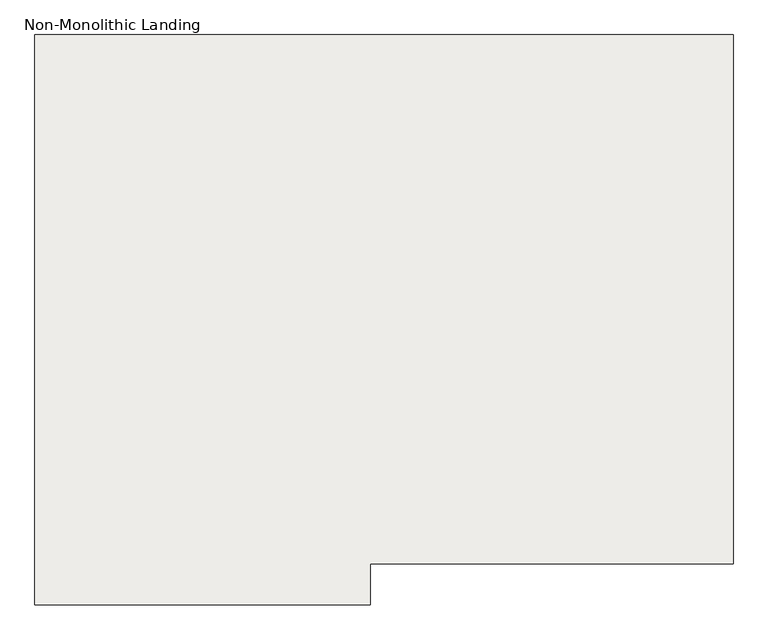
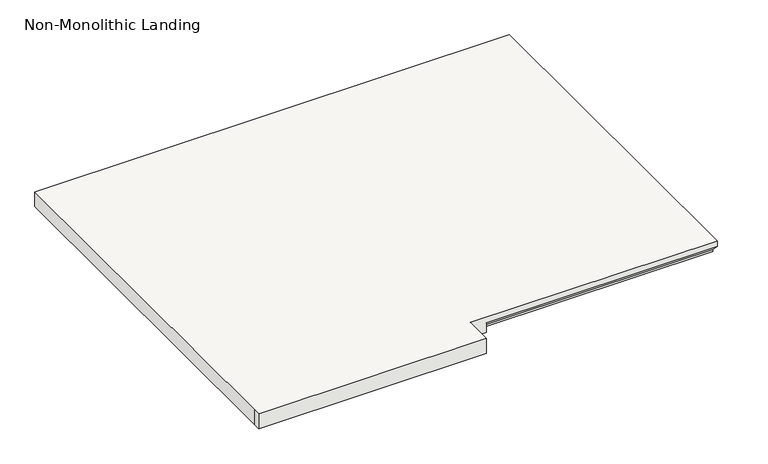
"""IFC4 building model written with IfcOpenShell, lengths in millimetres: slab geometry, Non-Monolithic Landing."""

from ifc_helpers import new_model, si_unit, origin, place, context, project, spatial, faceted_brep, source, transform, mapped, element, save


def non_monolithic_landing_83642a75(model_context):
    return source(origin(), model_context, "Body", "Brep", [
        faceted_brep([(-5330.5155596, 6109.0076853, 831.85), (-5330.5155596, 6083.6076853, 857.25), (-6072.1955596, 6083.6076853, 857.25), (-6072.1955596, 6109.0076853, 831.85), (-5330.5155596, 7239.3076853, 876.3), (-6854.5155596, 7239.3076853, 876.3), (-6854.5155596, 6020.1076853, 876.3), (-6854.5155596, 5994.7076853, 876.3), (-6122.9955596, 5994.7076853, 876.3), (-6122.9955596, 6020.1076853, 876.3), (-6122.9955596, 6083.6076853, 876.3), (-5330.5155596, 6083.6076853, 876.3), (-6072.1955596, 6109.0076853, 825.5), (-6072.1955596, 6083.6076853, 825.5), (-6122.9955596, 6083.6076853, 825.5), (-6122.9955596, 6020.1076853, 825.5), (-6122.9955596, 5994.7076853, 825.5), (-6854.5155596, 5994.7076853, 825.5), (-6854.5155596, 6020.1076853, 825.5), (-6854.5155596, 7239.3076853, 825.5), (-5330.5155596, 7239.3076853, 825.5), (-5330.5155596, 6109.0076853, 825.5)], [[[0, 1, 2, 3]], [[4, 5, 6, 7, 8, 9, 10, 11]], [[12, 13, 14, 15, 16, 17, 18, 19, 20, 21]], [[13, 12, 3, 2]], [[12, 21, 0, 3]], [[4, 11, 1, 0, 21, 20]], [[5, 4, 20, 19]], [[6, 5, 19, 18]], [[7, 6, 18, 17]], [[8, 7, 17, 16]], [[9, 8, 16, 15]], [[10, 9, 15, 14]], [[11, 10, 14, 13, 2, 1]]]),
    ])


if __name__ == "__main__":
    model = new_model("IFC4")
    model_context = context("Model", 3, world=origin())
    ifc_project = project(units=[si_unit("LENGTHUNIT", "METRE", prefix="MILLI")], contexts=[model_context])
    site = spatial("IfcSite", under=ifc_project)
    building = spatial("IfcBuilding", under=site)
    placement = place(None, origin())
    non_monolithic_landing_shape = non_monolithic_landing_83642a75(model_context)
    element("IfcSlab", 1, ObjectType="Non-Monolithic Landing", at=placement, inside=building, context=model_context, shape_type="MappedRepresentation", body=[
        mapped(non_monolithic_landing_shape, transform((0.0, 0.0, 0.0), x_axis=(1.0, 0.0, 0.0), y_axis=(0.0, 1.0, 0.0), z_axis=(0.0, 0.0, 1.0))),
    ])
    save(model, "model.ifc")
